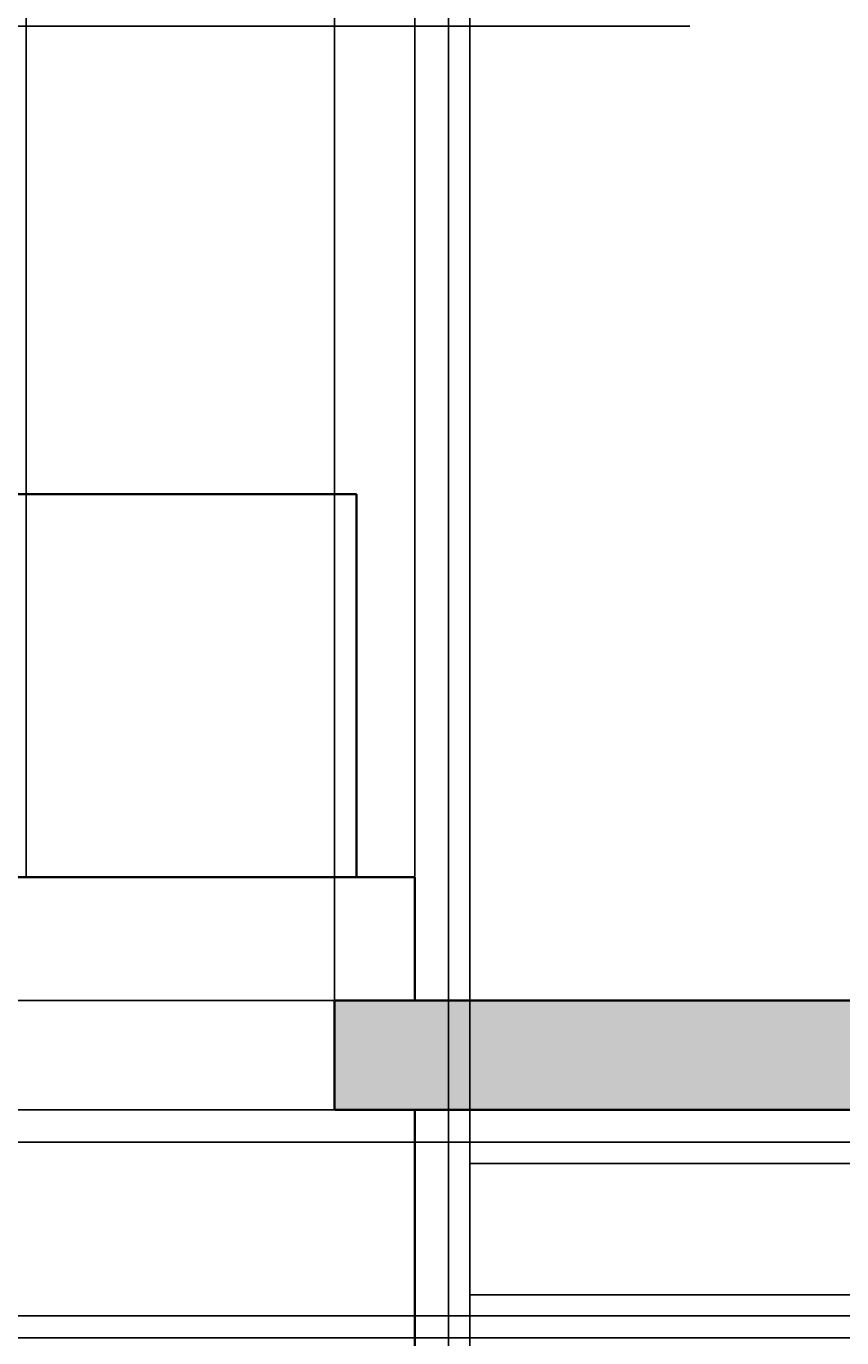
# Model space of a CAD drawing. Units: inches. Extents: x -145 to 510, y 5 to 386.
# Tile 19 of 25: x 182 to 259, y 157 to 280. Entities that reach past the tile are written whole.
import ezdxf

# ---------------------------------------------------------------- set-up
doc = ezdxf.new("R2010")
doc.units = ezdxf.units.IN
doc.header["$MEASUREMENT"] = 0
for name, color, linetype, lineweight in [('A-ANNO-DIMS', 2, 'Continuous', 18), ('A-ELEV', 7, 'Continuous', 35), ('A-ELEV-PATT', 8, 'Continuous', 13), ('A-GLAZ', 4, 'Continuous', 25)]:
    doc.layers.add(name, color=color, linetype=linetype, lineweight=lineweight)
doc.styles.get("Standard").update_dxf_attribs({"font": 'arial.ttf'})
doc.dimstyles.get("Standard").update_dxf_attribs({"dimtxt": 0.6875, "dimasz": 0.18, "dimexe": 0.18, "dimexo": 0.0625, "dimgap": 0.09, "dimtad": 0, "dimtih": 1, "dimtoh": 1, "dimdec": 4, "dimzin": 0, "dimdsep": 46, "dimlunit": 4, "dimtxsty": 'Standard', "dimcen": 0.09, "dimadec": 0, "dimazin": 0, "dimtfac": 1, "dimtdec": 4, "dimtofl": 0, "dimtmove": 0, "dimatfit": 3, "dimfxl": 1, "dimtolj": 1, "dimtzin": 0, "dimarcsym": 0})

# ---------------------------------------------------------------- blocks, each defined once
blk = doc.blocks.new('*D19')
at = {"layer": 'A-ANNO-DIMS', "color": 0, "lineweight": -2, "transparency": 16777216}
for p, q in [((478.76, 355.89), (-144.05, 355.89)), ((-143.87, 355.71), (-143.87, 218.33)), ((-143.87, 80.07), (-143.87, 217.45)), ((-114.04, 79.89), (-144.05, 79.89))]:
    blk.add_line(p, q, dxfattribs=at)
at = {"layer": 'A-ANNO-DIMS', "color": 0, "transparency": 16777216}
for points in [[(-143.9, 355.71), (-143.84, 355.71), (-143.87, 355.89)], [(-143.9, 80.07), (-143.84, 80.07), (-143.87, 79.89)]]:
    blk.add_solid(points, dxfattribs=at)
at = {"layer": 'Defpoints', "color": 0, "transparency": 16777216}
for p in [(-143.87, 355.89), (478.83, 355.89), (-113.97, 79.89)]:
    blk.add_point(p, dxfattribs=at)
at = {"layer": 'A-ANNO-DIMS', "color": 0, "transparency": 16777216, "insert": (-143.87, 217.89), "char_height": 0.688, "attachment_point": 5}
blk.add_mtext('\\A1;276', dxfattribs=at)
blk = doc.blocks.new('*D27')
at = {"layer": 'A-ANNO-DIMS', "color": 0, "lineweight": -2, "transparency": 16777216}
for p, q in [((244.23, 279.84), (-144.05, 279.84)), ((-143.87, 279.66), (-143.87, 240.31)), ((-143.87, 200.07), (-143.87, 239.43)), ((218.29, 199.89), (-144.05, 199.89))]:
    blk.add_line(p, q, dxfattribs=at)
at = {"layer": 'A-ANNO-DIMS', "color": 0, "transparency": 16777216}
for points in [[(-143.9, 279.66), (-143.84, 279.66), (-143.87, 279.84)], [(-143.9, 200.07), (-143.84, 200.07), (-143.87, 199.89)]]:
    blk.add_solid(points, dxfattribs=at)
at = {"layer": 'Defpoints', "color": 0, "transparency": 16777216}
for p in [(-143.87, 279.84), (244.29, 279.84), (218.36, 199.89)]:
    blk.add_point(p, dxfattribs=at)
at = {"layer": 'A-ANNO-DIMS', "color": 0, "transparency": 16777216, "insert": (-143.87, 239.87), "char_height": 0.688, "attachment_point": 5}
blk.add_mtext('\\A1;79.95', dxfattribs=at)
blk = doc.blocks.new('*D28')
at = {"layer": 'A-ANNO-DIMS', "color": 0, "lineweight": -2, "transparency": 16777216}
for p, q in [((244.23, 305.74), (-144.05, 305.74)), ((-143.87, 305.56), (-143.87, 293.23)), ((-143.87, 280.02), (-143.87, 292.35)), ((244.23, 279.84), (-144.05, 279.84))]:
    blk.add_line(p, q, dxfattribs=at)
at = {"layer": 'A-ANNO-DIMS', "color": 0, "transparency": 16777216}
for points in [[(-143.9, 305.56), (-143.84, 305.56), (-143.87, 305.74)], [(-143.9, 280.02), (-143.84, 280.02), (-143.87, 279.84)]]:
    blk.add_solid(points, dxfattribs=at)
at = {"layer": 'Defpoints', "color": 0, "transparency": 16777216}
for p in [(-143.87, 305.74), (244.29, 305.74), (244.29, 279.84)]:
    blk.add_point(p, dxfattribs=at)
at = {"layer": 'A-ANNO-DIMS', "color": 0, "transparency": 16777216, "insert": (-143.87, 292.79), "char_height": 0.688, "attachment_point": 5}
blk.add_mtext('\\A1;25.897', dxfattribs=at)
blk = doc.blocks.new('*D29')
at = {"layer": 'A-ANNO-DIMS', "color": 0, "lineweight": -2, "transparency": 16777216}
for p, q in [((221.47, 174.99), (-144.05, 174.99)), ((-143.87, 174.81), (-143.87, 130.57)), ((-143.87, 85.44), (-143.87, 129.69)), ((221.47, 85.26), (-144.05, 85.26))]:
    blk.add_line(p, q, dxfattribs=at)
at = {"layer": 'A-ANNO-DIMS', "color": 0, "transparency": 16777216}
for points in [[(-143.9, 174.81), (-143.84, 174.81), (-143.87, 174.99)], [(-143.9, 85.44), (-143.84, 85.44), (-143.87, 85.26)]]:
    blk.add_solid(points, dxfattribs=at)
at = {"layer": 'Defpoints', "color": 0, "transparency": 16777216}
for p in [(-143.87, 174.99), (221.53, 174.99), (221.53, 85.26)]:
    blk.add_point(p, dxfattribs=at)
at = {"layer": 'A-ANNO-DIMS', "color": 0, "transparency": 16777216, "insert": (-143.87, 130.13), "char_height": 0.688, "attachment_point": 5}
blk.add_mtext('\\A1;89.73', dxfattribs=at)
blk = doc.blocks.new('*D30')
at = {"layer": 'A-ANNO-DIMS', "color": 0, "lineweight": -2, "transparency": 16777216}
for p, q in [((210.73, 188.31), (-144.05, 188.31)), ((-143.87, 188.13), (-143.87, 183.61)), ((-143.87, 178.2), (-143.87, 182.72)), ((210.73, 178.02), (-144.05, 178.02))]:
    blk.add_line(p, q, dxfattribs=at)
at = {"layer": 'A-ANNO-DIMS', "color": 0, "transparency": 16777216}
for points in [[(-143.9, 188.13), (-143.84, 188.13), (-143.87, 188.31)], [(-143.9, 178.2), (-143.84, 178.2), (-143.87, 178.02)]]:
    blk.add_solid(points, dxfattribs=at)
at = {"layer": 'Defpoints', "color": 0, "transparency": 16777216}
for p in [(-143.87, 188.31), (210.8, 188.31), (210.8, 178.02)]:
    blk.add_point(p, dxfattribs=at)
at = {"layer": 'A-ANNO-DIMS', "color": 0, "transparency": 16777216, "insert": (-143.87, 183.16), "char_height": 0.688, "attachment_point": 5}
blk.add_mtext('\\A1;10.29', dxfattribs=at)
blk = doc.blocks.new('*D45')
at = {"layer": 'A-ANNO-DIMS', "color": 0, "lineweight": -2, "transparency": 16777216}
for p, q in [((210.8, 188.37), (210.8, 385.97)), ((210.98, 385.79), (262.53, 385.79)), ((317.05, 385.79), (265.5, 385.79)), ((317.23, 178.08), (317.23, 385.97))]:
    blk.add_line(p, q, dxfattribs=at)
at = {"layer": 'A-ANNO-DIMS', "color": 0, "transparency": 16777216}
for points in [[(210.98, 385.82), (210.98, 385.76), (210.8, 385.79)], [(317.05, 385.82), (317.05, 385.76), (317.23, 385.79)]]:
    blk.add_solid(points, dxfattribs=at)
at = {"layer": 'Defpoints', "color": 0, "transparency": 16777216}
for p in [(317.23, 385.79), (210.8, 188.31), (317.23, 178.02)]:
    blk.add_point(p, dxfattribs=at)
at = {"layer": 'A-ANNO-DIMS', "color": 0, "transparency": 16777216, "insert": (264.01, 385.79), "char_height": 0.688, "attachment_point": 5}
blk.add_mtext('\\A1;106.43', dxfattribs=at)
blk = doc.blocks.new('*D46')
at = {"layer": 'A-ANNO-DIMS', "color": 0, "lineweight": -2, "transparency": 16777216}
for p, q in [((181.82, 199.95), (181.82, 385.97)), ((182, 385.79), (198.84, 385.79)), ((218.18, 385.79), (201.34, 385.79)), ((218.36, 199.95), (218.36, 385.97))]:
    blk.add_line(p, q, dxfattribs=at)
at = {"layer": 'A-ANNO-DIMS', "color": 0, "transparency": 16777216}
for points in [[(182, 385.82), (182, 385.76), (181.82, 385.79)], [(218.18, 385.82), (218.18, 385.76), (218.36, 385.79)]]:
    blk.add_solid(points, dxfattribs=at)
at = {"layer": 'Defpoints', "color": 0, "transparency": 16777216}
for p in [(218.36, 385.79), (181.82, 199.89), (218.36, 199.89)]:
    blk.add_point(p, dxfattribs=at)
at = {"layer": 'A-ANNO-DIMS', "color": 0, "transparency": 16777216, "insert": (200.09, 385.79), "char_height": 0.688, "attachment_point": 5}
blk.add_mtext('\\A1;36.54', dxfattribs=at)
blk = doc.blocks.new('*D50')
at = {"layer": 'A-ANNO-DIMS', "color": 0, "lineweight": -2, "transparency": 16777216}
for p, q in [((221.53, 156.67), (221.53, 385.97)), ((221.71, 385.79), (246.26, 385.79)), ((273.31, 385.79), (248.76, 385.79)), ((273.49, 156.67), (273.49, 385.97))]:
    blk.add_line(p, q, dxfattribs=at)
at = {"layer": 'A-ANNO-DIMS', "color": 0, "transparency": 16777216}
for points in [[(221.71, 385.82), (221.71, 385.76), (221.53, 385.79)], [(273.31, 385.82), (273.31, 385.76), (273.49, 385.79)]]:
    blk.add_solid(points, dxfattribs=at)
at = {"layer": 'Defpoints', "color": 0, "transparency": 16777216}
for p in [(273.49, 385.79), (221.53, 156.61), (273.49, 156.61)]:
    blk.add_point(p, dxfattribs=at)
at = {"layer": 'A-ANNO-DIMS', "color": 0, "transparency": 16777216, "insert": (247.51, 385.79), "char_height": 0.688, "attachment_point": 5}
blk.add_mtext('\\A1;51.96', dxfattribs=at)
blk = doc.blocks.new('*D53')
at = {"layer": 'A-ANNO-DIMS', "color": 0, "lineweight": -2, "transparency": 16777216}
for p, q in [((221.53, 85.33), (221.53, 385.97)), ((221.71, 385.79), (222.21, 385.79)), ((223.35, 385.79), (222.85, 385.79)), ((223.53, 87.33), (223.53, 385.97))]:
    blk.add_line(p, q, dxfattribs=at)
at = {"layer": 'A-ANNO-DIMS', "color": 0, "transparency": 16777216}
for points in [[(221.71, 385.82), (221.71, 385.76), (221.53, 385.79)], [(223.35, 385.82), (223.35, 385.76), (223.53, 385.79)]]:
    blk.add_solid(points, dxfattribs=at)
at = {"layer": 'Defpoints', "color": 0, "transparency": 16777216}
for p in [(223.53, 385.79), (223.53, 87.26), (221.53, 85.26)]:
    blk.add_point(p, dxfattribs=at)
at = {"layer": 'A-ANNO-DIMS', "color": 0, "transparency": 16777216, "insert": (222.53, 385.79), "char_height": 0.688, "attachment_point": 5}
blk.add_mtext('\\A1;2', dxfattribs=at)
blk = doc.blocks.new('*D54')
at = {"layer": 'A-ANNO-DIMS', "color": 0, "lineweight": -2, "transparency": 16777216}
for p, q in [((315.49, 156.61), (-144.05, 156.61)), ((-143.87, 156.43), (-143.87, 121.38)), ((-143.87, 85.44), (-143.87, 120.5)), ((315.49, 85.26), (-144.05, 85.26))]:
    blk.add_line(p, q, dxfattribs=at)
at = {"layer": 'A-ANNO-DIMS', "color": 0, "transparency": 16777216}
for points in [[(-143.9, 156.43), (-143.84, 156.43), (-143.87, 156.61)], [(-143.9, 85.44), (-143.84, 85.44), (-143.87, 85.26)]]:
    blk.add_solid(points, dxfattribs=at)
at = {"layer": 'Defpoints', "color": 0, "transparency": 16777216}
for p in [(-143.87, 156.61), (315.55, 156.61), (315.55, 85.26)]:
    blk.add_point(p, dxfattribs=at)
at = {"layer": 'A-ANNO-DIMS', "color": 0, "transparency": 16777216, "insert": (-143.87, 120.94), "char_height": 0.688, "attachment_point": 5}
blk.add_mtext('\\A1;71.35', dxfattribs=at)
blk = doc.blocks.new('*D55')
at = {"layer": 'A-ANNO-DIMS', "color": 0, "lineweight": -2, "transparency": 16777216}
for p, q in [((314.43, 174.99), (-144.05, 174.99)), ((-143.87, 174.81), (-143.87, 167.27)), ((-143.87, 158.84), (-143.87, 166.38)), ((314.43, 158.66), (-144.05, 158.66))]:
    blk.add_line(p, q, dxfattribs=at)
at = {"layer": 'A-ANNO-DIMS', "color": 0, "transparency": 16777216}
for points in [[(-143.9, 174.81), (-143.84, 174.81), (-143.87, 174.99)], [(-143.9, 158.84), (-143.84, 158.84), (-143.87, 158.66)]]:
    blk.add_solid(points, dxfattribs=at)
at = {"layer": 'Defpoints', "color": 0, "transparency": 16777216}
for p in [(-143.87, 174.99), (314.49, 174.99), (314.49, 158.66)]:
    blk.add_point(p, dxfattribs=at)
at = {"layer": 'A-ANNO-DIMS', "color": 0, "transparency": 16777216, "insert": (-143.87, 166.82), "char_height": 0.688, "attachment_point": 5}
blk.add_mtext('\\A1;16.335', dxfattribs=at)

msp = doc.modelspace()

# ---------------------------------------------------------------- hatches: boundary and pattern name
at = {"layer": 'A-ELEV-PATT'}
h = msp.add_hatch(color=256, dxfattribs=at)
h.dxf.hatch_style = 1
h.paths.add_polyline_path([(334.4402, 341.168), (69.7763, 341.168), (69.7763, 327.6093), (334.4402, 327.6093)])
h.paths.add_polyline_path([(69.7763, 341.168), (34.2706, 341.168), (34.2706, 327.6093), (69.7763, 327.6093)])
h.paths.add_polyline_path([(317.2273, 188.3087), (210.7973, 188.3087), (210.7973, 178.0195), (317.2273, 178.0195)])
h.paths.add_polyline_path([(474.4893, 235.8905), (317.2273, 235.8905), (317.2273, 223.8905), (474.4893, 223.8905)])
h.paths.add_polyline_path([(317.2273, 235.8905), (309.4739, 235.8905), (309.4739, 223.8905), (317.2273, 223.8905)])
h.paths.add_polyline_path([(478.8263, 235.8905), (474.4893, 235.8905), (474.4893, 223.8905), (478.8263, 223.8905)])

# ---------------------------------------------------------------- linework, layer by layer
at = {"layer": 'A-ELEV'}
for p, q in [((74.5073, 235.8905), (212.8652, 235.8905)), ((212.8652, 235.8905), (212.8652, 199.8905)), ((218.3571, 199.8905), (54.0014, 199.8905)), ((218.3571, 199.8905), (218.3571, 188.3087)), ((210.7973, 188.3087), (317.2273, 188.3087)), ((210.7973, 188.3087), (210.7973, 178.0195)), ((210.7973, 178.0195), (317.2273, 178.0195)), ((218.3571, 178.0195), (218.3571, 79.8905))]:
    msp.add_line(p, q, dxfattribs=at)
at = {"layer": 'A-GLAZ'}
for points in [[(221.5292, 174.9923), (314.494, 174.9923), (314.494, 158.657), (221.5292, 158.657)], [(223.5292, 172.9923), (312.494, 172.9923), (312.494, 160.657), (223.5292, 160.657)]]:
    msp.add_lwpolyline(points, close=True, dxfattribs=at)

# ---------------------------------------------------------------- dimensions: what is measured, and where the dimension line sits
at = {"layer": 'A-ANNO-DIMS'}
for base, p1, p2, override, picture, middle in [((218.3571, 385.7905), (181.8195, 199.8905), (218.3571, 199.8905), {"dimdec": 2, "dimlfac": 1, "dimrnd": 0, "dimzin": 0, "dimdsep": 46, "dimlunit": 2}, '*D46', (200.0883, 385.7905)), ((317.2273, 385.7905), (210.7973, 188.3087), (317.2273, 178.0195), {"dimdec": 2, "dimlfac": 1, "dimrnd": 0, "dimzin": 0, "dimdsep": 46, "dimlunit": 2}, '*D45', (264.0123, 385.7905)), ((273.4905, 385.7905), (221.5292, 156.6093), (273.4905, 156.6093), {"dimdec": 2, "dimlfac": 1, "dimrnd": 0, "dimzin": 0, "dimdsep": 46, "dimlunit": 2}, '*D50', (247.5098, 385.7905)), ((223.5292, 385.7905), (221.5292, 85.2638), (223.5292, 87.2638), {"dimdec": 0, "dimlfac": 1, "dimrnd": 0, "dimzin": 0, "dimdsep": 46, "dimlunit": 2}, '*D53', (222.5292, 385.7905))]:
    dim = msp.add_linear_dim(base=base, p1=p1, p2=p2, dimstyle='Standard', override=override, dxfattribs=at)
    dim.commit()
    dim.dimension.update_dxf_attribs({"geometry": picture, "text_midpoint": middle})
for base, p1, p2, override, picture, middle in [((-143.8737, 355.8905), (-113.9737, 79.8905), (478.8263, 355.8905), {"dimdec": 0, "dimlfac": 1, "dimrnd": 0, "dimzin": 0, "dimdsep": 46, "dimlunit": 2}, '*D19', (-143.8737, 217.8905)), ((-143.8737, 305.7416), (244.2916, 279.8443), (244.2916, 305.7416), {"dimdec": 3, "dimlfac": 1, "dimrnd": 0, "dimzin": 0, "dimdsep": 46, "dimlunit": 2}, '*D28', (-143.8737, 292.793)), ((-143.8737, 279.8443), (218.3571, 199.8905), (244.2916, 279.8443), {"dimdec": 2, "dimlfac": 1, "dimrnd": 0, "dimzin": 0, "dimdsep": 46, "dimlunit": 2}, '*D27', (-143.8737, 239.8674)), ((-143.8737, 188.3087), (210.7973, 178.0195), (210.7973, 188.3087), {"dimdec": 2, "dimlfac": 1, "dimrnd": 0, "dimzin": 0, "dimdsep": 46, "dimlunit": 2}, '*D30', (-143.8737, 183.1641)), ((-143.8737, 174.9923), (314.494, 158.657), (314.494, 174.9923), {"dimdec": 3, "dimlfac": 1, "dimrnd": 0, "dimzin": 0, "dimdsep": 46, "dimlunit": 2}, '*D55', (-143.8737, 166.8247)), ((-143.8737, 174.9923), (221.5292, 85.2638), (221.5292, 174.9923), {"dimdec": 2, "dimlfac": 1, "dimrnd": 0, "dimzin": 0, "dimdsep": 46, "dimlunit": 2}, '*D29', (-143.8737, 130.1281)), ((-143.8737, 156.6093), (315.5545, 85.2638), (315.5545, 156.6093), {"dimdec": 2, "dimlfac": 1, "dimrnd": 0, "dimzin": 0, "dimdsep": 46, "dimlunit": 2}, '*D54', (-143.8737, 120.9365))]:
    dim = msp.add_linear_dim(base=base, p1=p1, p2=p2, angle=90, dimstyle='Standard', override=override, dxfattribs=at)
    dim.commit()
    dim.dimension.update_dxf_attribs({"geometry": picture, "text_midpoint": middle})

doc.saveas('drawing.dxf')
